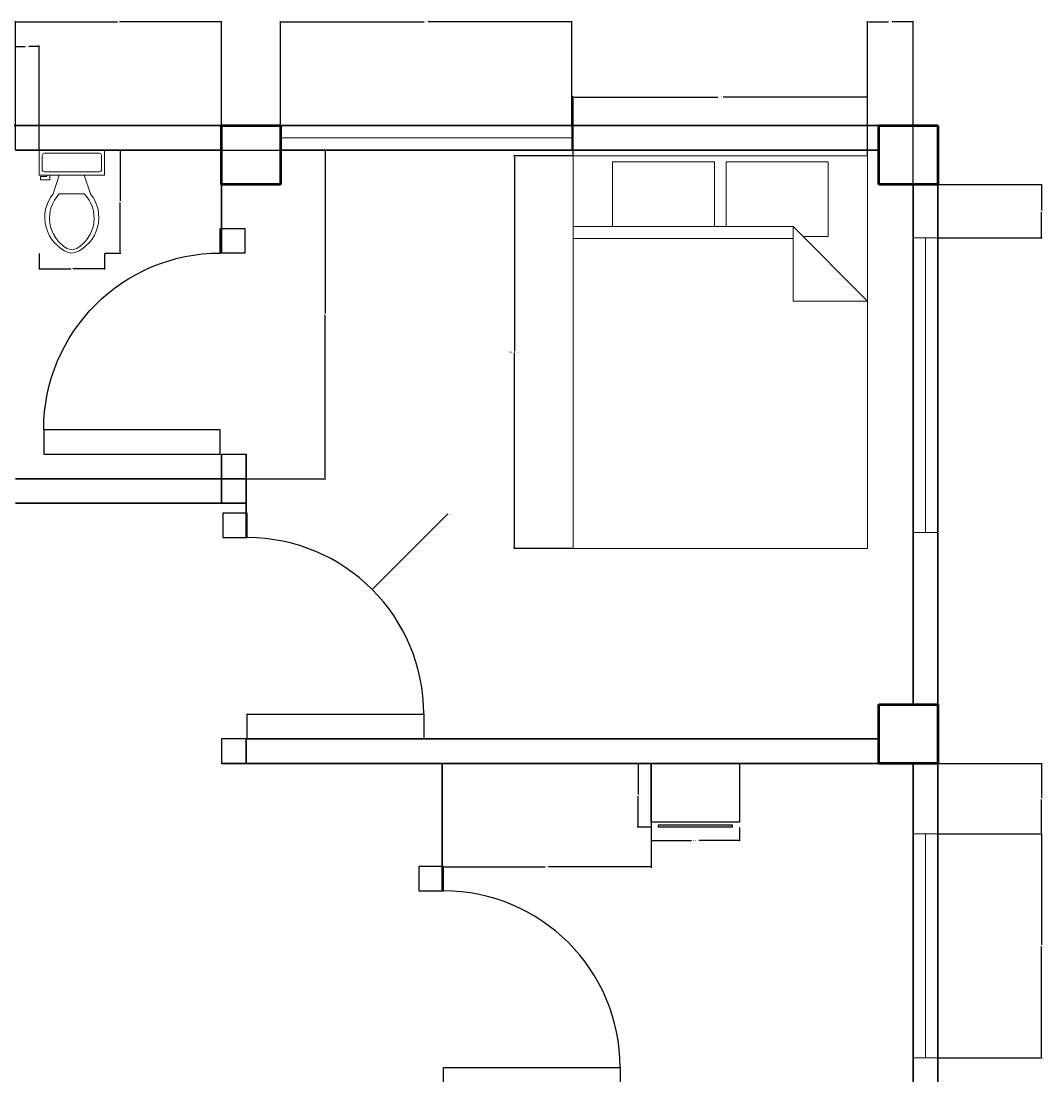
# Model space of a CAD drawing. Units: inches. Extents: x 2082 to 2506, y 790 to 1201.
# Tile 3 of 3: x 2298 to 2506, y 986 to 1201. Entities that reach past the tile are written whole.
import ezdxf

# ---------------------------------------------------------------- set-up
doc = ezdxf.new("R2010")
doc.units = ezdxf.units.IN
for name, color, linetype, lineweight in [('A-ANNO-DIMS', 2, 'Continuous', 18), ('A-COLS', 7, 'Continuous', 50), ('A-DOOR', 3, 'Continuous', 25), ('A-FLOR-CASE', 8, 'Continuous', 25), ('A-FLOR-FIXT', 9, 'Continuous', 18), ('A-FURN', 8, 'Continuous', 18), ('A-GLAZ', 4, 'Continuous', 18), ('A-WALL', 7, 'Continuous', 35)]:
    doc.layers.add(name, color=color, linetype=linetype, lineweight=lineweight)
doc.styles.get("Standard").update_dxf_attribs({"font": 'arial.ttf'})
doc.dimstyles.get("Standard").update_dxf_attribs({"dimtxt": 0.18, "dimasz": 0.18, "dimexe": 0.18, "dimexo": 0.0625, "dimgap": 0.09, "dimtad": 0, "dimtih": 1, "dimtoh": 1, "dimdec": 4, "dimzin": 0, "dimdsep": 46, "dimlunit": 4, "dimtxsty": 'Standard', "dimcen": 0.09, "dimadec": 0, "dimazin": 0, "dimtfac": 1, "dimtdec": 4, "dimtofl": 0, "dimtmove": 0, "dimatfit": 3, "dimfxl": 1, "dimtolj": 1, "dimtzin": 0, "dimarcsym": 0})

# ---------------------------------------------------------------- blocks, each defined once
blk = doc.blocks.new('Wall Cabinet - 18 x 12 in side')
for points in [[(-12, -18), (-12, 0), (0, 0), (0, -18)], [(-13, -16.5), (-13, -1.5), (-12.5, -1.5), (-12.5, -16.5)]]:
    blk.add_lwpolyline(points, close=True)
blk = doc.blocks.new('Toilet - top')
for p, q in [((9.5, -6), (9.5, -2)), ((-10, -8.5), (-8, -8.5)), ((-10, -9.5), (-10, -8.5)), ((-7, -9.5), (-10, -9.5)), ((-8, -8.5), (-8, -8)), ((-7, -8), (-7, -9.5)), ((-4, -8), (-6, -14)), ((4, -8), (6, -14)), ((4, -14), (-4, -14))]:
    blk.add_line(p, q)
blk.add_lwpolyline([(10.5, -8), (10.5, 0), (-10.5, 0), (-10.5, -8)], close=True)
for points in [[(-9.5, -2), (-9.5, -6)], [(8.5, -1), (-8.5, -1)], [(-8.5, -7), (8.5, -7)]]:
    blk.add_lwpolyline(points)
for centre, radius, start, end in [((-8.62, -1.88), 0.884, 81.8699, 188.1301), ((8.62, -1.88), 0.884, 351.8699, 98.1301), ((-8.62, -6.12), 0.884, 171.8699, 278.1301), ((8.62, -6.12), 0.884, 261.8699, 8.1301), ((3.52, -21.58), 12.17, 141.4691, 247.9714), ((4.2, -21.82), 11.33, 136.3677, 238.9468), ((-3.52, -21.58), 12.17, 292.0284, 38.5307), ((-4.2, -21.82), 11.33, 301.053, 43.6321), ((0, -27.88), 4, 245.7318, 294.2682), ((0, -29), 4, 254.8605, 285.1395)]:
    blk.add_arc(centre, radius, start, end)
blk = doc.blocks.new('Bed - Queen')
for p, q in [((0, -80.00003), (0, 0)), ((0, 0), (59.99999, 0)), ((59.99999, 0), (59.99999, -80.00003)), ((7.99999, -1.2), (28.79998, -1.2)), ((7.99999, -14.4), (7.99999, -1.2)), ((28.79998, -1.2), (28.79998, -14.4)), ((31.19999, -1.2), (51.99999, -1.2)), ((31.19999, -14.4), (31.19999, -1.2)), ((51.99999, -1.2), (51.99999, -16.4)), ((0, -14.4), (44.8, -14.4)), ((59.99999, -29.6), (44.8, -14.4)), ((44.8, -14.4), (44.8, -29.6)), ((44.8, -16.8), (0, -16.8)), ((51.99999, -16.4), (46.79936, -16.4)), ((44.8, -29.6), (59.99999, -29.6)), ((59.99999, -80.00003), (0, -80.00003))]:
    blk.add_line(p, q)
blk = doc.blocks.new('DOOR-SWING-36IN')
for p, q in [((0, 0), (0, 5)), ((0, 5), (36, 5)), ((36, 5), (36, 0)), ((36, 0), (0, 0))]:
    blk.add_line(p, q)
blk.add_arc((0, 5), 36, 0, 90)
blk = doc.blocks.new('WIN-60IN')
for p, q in [((0, 5), (12, 5)), ((0, 5), (0, 0)), ((12, 5), (60, 5)), ((60, 5), (60, 0)), ((0, 2.5), (60, 2.5)), ((0, 0), (60, 0))]:
    blk.add_line(p, q)
blk = doc.blocks.new('COL-12X12IN')
for p, q in [((0, 12), (12, 12)), ((0, 0), (0, 12)), ((12, 12), (12, 0)), ((12, 0), (0, 0))]:
    blk.add_line(p, q)
blk = doc.blocks.new('*D10')
at = {"layer": 'A-ANNO-DIMS', "color": 0, "lineweight": -2, "transparency": 16777216}
for p, q in [((2410.56, 1173.3), (2398.44, 1173.3)), ((2398.62, 1173.12), (2398.62, 1133.49)), ((2398.62, 1093.48), (2398.62, 1133.11)), ((2410.56, 1093.3), (2398.44, 1093.3))]:
    blk.add_line(p, q, dxfattribs=at)
at = {"layer": 'A-ANNO-DIMS', "color": 0, "transparency": 16777216}
for points in [[(2398.59, 1173.12), (2398.65, 1173.12), (2398.62, 1173.3)], [(2398.59, 1093.48), (2398.65, 1093.48), (2398.62, 1093.3)]]:
    blk.add_solid(points, dxfattribs=at)
at = {"layer": 'Defpoints', "color": 0, "transparency": 16777216}
for p in [(2398.62, 1173.3), (2410.62, 1173.3), (2410.62, 1093.3)]:
    blk.add_point(p, dxfattribs=at)
at = {"layer": 'A-ANNO-DIMS', "color": 0, "transparency": 16777216, "insert": (2398.62, 1133.3), "char_height": 0.18, "attachment_point": 5}
blk.add_mtext('\\A1;QUEEN BED 80 TYP.', dxfattribs=at)
blk = doc.blocks.new('*D11')
at = {"layer": 'A-ANNO-DIMS', "color": 0, "lineweight": -2, "transparency": 16777216}
for p, q in [((2410.62, 1173.36), (2410.62, 1185.48)), ((2410.8, 1185.3), (2440.09, 1185.3)), ((2470.44, 1185.3), (2441.15, 1185.3)), ((2470.62, 1173.36), (2470.62, 1185.48))]:
    blk.add_line(p, q, dxfattribs=at)
at = {"layer": 'A-ANNO-DIMS', "color": 0, "transparency": 16777216}
for points in [[(2410.8, 1185.33), (2410.8, 1185.27), (2410.62, 1185.3)], [(2470.44, 1185.33), (2470.44, 1185.27), (2470.62, 1185.3)]]:
    blk.add_solid(points, dxfattribs=at)
at = {"layer": 'Defpoints', "color": 0, "transparency": 16777216}
for p in [(2470.62, 1185.3), (2410.62, 1173.3), (2470.62, 1173.3)]:
    blk.add_point(p, dxfattribs=at)
at = {"layer": 'A-ANNO-DIMS', "color": 0, "transparency": 16777216, "insert": (2440.62, 1185.3), "char_height": 0.18, "attachment_point": 5}
blk.add_mtext('\\A1;60 TYP.', dxfattribs=at)
blk = doc.blocks.new('*D18')
at = {"layer": 'A-ANNO-DIMS', "color": 0, "lineweight": -2, "transparency": 16777216}
for p, q in [((2315.16, 1174.5), (2318.43, 1174.5)), ((2318.25, 1174.32), (2318.25, 1164.17)), ((2318.25, 1153.65), (2318.25, 1163.8)), ((2315.16, 1153.47), (2318.43, 1153.47))]:
    blk.add_line(p, q, dxfattribs=at)
at = {"layer": 'A-ANNO-DIMS', "color": 0, "transparency": 16777216}
for points in [[(2318.22, 1174.32), (2318.28, 1174.32), (2318.25, 1174.5)], [(2318.22, 1153.65), (2318.28, 1153.65), (2318.25, 1153.47)]]:
    blk.add_solid(points, dxfattribs=at)
at = {"layer": 'Defpoints', "color": 0, "transparency": 16777216}
for p in [(2315.09, 1174.5), (2318.25, 1174.5), (2315.09, 1153.47)]:
    blk.add_point(p, dxfattribs=at)
at = {"layer": 'A-ANNO-DIMS', "color": 0, "transparency": 16777216, "insert": (2318.25, 1163.98), "char_height": 0.18, "attachment_point": 5}
blk.add_mtext('\\A1;WC 21', dxfattribs=at)
blk = doc.blocks.new('*D19')
at = {"layer": 'A-ANNO-DIMS', "color": 0, "lineweight": -2, "transparency": 16777216}
for p, q in [((2301.73, 1153.4), (2301.73, 1150.13)), ((2315.09, 1153.4), (2315.09, 1150.13)), ((2301.91, 1150.31), (2308.2, 1150.31)), ((2314.91, 1150.31), (2308.62, 1150.31))]:
    blk.add_line(p, q, dxfattribs=at)
at = {"layer": 'A-ANNO-DIMS', "color": 0, "transparency": 16777216}
for points in [[(2301.91, 1150.34), (2301.91, 1150.28), (2301.73, 1150.31)], [(2314.91, 1150.34), (2314.91, 1150.28), (2315.09, 1150.31)]]:
    blk.add_solid(points, dxfattribs=at)
at = {"layer": 'Defpoints', "color": 0, "transparency": 16777216}
for p in [(2301.73, 1153.47), (2315.09, 1153.47), (2315.09, 1150.31)]:
    blk.add_point(p, dxfattribs=at)
at = {"layer": 'A-ANNO-DIMS', "color": 0, "transparency": 16777216, "insert": (2308.41, 1150.31), "char_height": 0.18, "attachment_point": 5}
blk.add_mtext('\\A1;13', dxfattribs=at)
blk = doc.blocks.new('*D20')
at = {"layer": 'A-ANNO-DIMS', "color": 0, "lineweight": -2, "transparency": 16777216}
for p, q in [((2426.53, 1036.44), (2426.53, 1033.62)), ((2444.53, 1036.44), (2444.53, 1033.62)), ((2426.71, 1033.8), (2434.73, 1033.8)), ((2444.35, 1033.8), (2436.32, 1033.8))]:
    blk.add_line(p, q, dxfattribs=at)
at = {"layer": 'A-ANNO-DIMS', "color": 0, "transparency": 16777216}
for points in [[(2426.71, 1033.83), (2426.71, 1033.77), (2426.53, 1033.8)], [(2444.35, 1033.83), (2444.35, 1033.77), (2444.53, 1033.8)]]:
    blk.add_solid(points, dxfattribs=at)
at = {"layer": 'Defpoints', "color": 0, "transparency": 16777216}
for p in [(2426.53, 1036.5), (2444.53, 1036.5), (2426.53, 1033.8)]:
    blk.add_point(p, dxfattribs=at)
at = {"layer": 'A-ANNO-DIMS', "color": 0, "transparency": 16777216, "insert": (2435.53, 1033.8), "char_height": 0.18, "attachment_point": 5}
blk.add_mtext('\\A1;CABINET 18', dxfattribs=at)
blk = doc.blocks.new('*D21')
at = {"layer": 'A-ANNO-DIMS', "color": 0, "lineweight": -2, "transparency": 16777216}
for p, q in [((2426.46, 1049.5), (2423.65, 1049.5)), ((2423.83, 1049.32), (2423.83, 1043.18)), ((2423.83, 1036.68), (2423.83, 1042.82)), ((2426.46, 1036.5), (2423.65, 1036.5))]:
    blk.add_line(p, q, dxfattribs=at)
at = {"layer": 'A-ANNO-DIMS', "color": 0, "transparency": 16777216}
for points in [[(2423.8, 1049.32), (2423.86, 1049.32), (2423.83, 1049.5)], [(2423.8, 1036.68), (2423.86, 1036.68), (2423.83, 1036.5)]]:
    blk.add_solid(points, dxfattribs=at)
at = {"layer": 'Defpoints', "color": 0, "transparency": 16777216}
for p in [(2423.83, 1049.5), (2426.53, 1049.5), (2426.53, 1036.5)]:
    blk.add_point(p, dxfattribs=at)
at = {"layer": 'A-ANNO-DIMS', "color": 0, "transparency": 16777216, "insert": (2423.83, 1043), "char_height": 0.18, "attachment_point": 5}
blk.add_mtext('\\A1;13', dxfattribs=at)
blk = doc.blocks.new('*D33')
at = {"layer": 'A-ANNO-DIMS', "color": 0, "lineweight": -2, "transparency": 16777216}
for p, q in [((2296.92, 1174.56), (2296.92, 1200.78)), ((2338.92, 1174.56), (2338.92, 1200.78)), ((2297.1, 1200.6), (2317.7, 1200.6)), ((2338.74, 1200.6), (2318.15, 1200.6))]:
    blk.add_line(p, q, dxfattribs=at)
at = {"layer": 'A-ANNO-DIMS', "color": 0, "transparency": 16777216}
for points in [[(2297.1, 1200.63), (2297.1, 1200.57), (2296.92, 1200.6)], [(2338.74, 1200.63), (2338.74, 1200.57), (2338.92, 1200.6)]]:
    blk.add_solid(points, dxfattribs=at)
at = {"layer": 'Defpoints', "color": 0, "transparency": 16777216}
for p in [(2338.92, 1200.6), (2296.92, 1174.5), (2338.92, 1174.5)]:
    blk.add_point(p, dxfattribs=at)
at = {"layer": 'A-ANNO-DIMS', "color": 0, "transparency": 16777216, "insert": (2317.92, 1200.6), "char_height": 0.18, "attachment_point": 5}
blk.add_mtext('\\A1;42', dxfattribs=at)
blk = doc.blocks.new('*D34')
at = {"layer": 'A-ANNO-DIMS', "color": 0, "lineweight": -2, "transparency": 16777216}
for p, q in [((2350.92, 1179.56), (2350.92, 1200.78)), ((2410.34, 1179.56), (2410.34, 1200.78)), ((2351.1, 1200.6), (2380.24, 1200.6)), ((2410.16, 1200.6), (2381.02, 1200.6))]:
    blk.add_line(p, q, dxfattribs=at)
at = {"layer": 'A-ANNO-DIMS', "color": 0, "transparency": 16777216}
for points in [[(2351.1, 1200.63), (2351.1, 1200.57), (2350.92, 1200.6)], [(2410.16, 1200.63), (2410.16, 1200.57), (2410.34, 1200.6)]]:
    blk.add_solid(points, dxfattribs=at)
at = {"layer": 'Defpoints', "color": 0, "transparency": 16777216}
for p in [(2410.34, 1200.6), (2350.92, 1179.5), (2410.34, 1179.5)]:
    blk.add_point(p, dxfattribs=at)
at = {"layer": 'A-ANNO-DIMS', "color": 0, "transparency": 16777216, "insert": (2380.63, 1200.6), "char_height": 0.18, "attachment_point": 5}
blk.add_mtext('\\A1;59.42', dxfattribs=at)
blk = doc.blocks.new('*D35')
at = {"layer": 'A-ANNO-DIMS', "color": 0, "lineweight": -2, "transparency": 16777216}
for p, q in [((2338.99, 1174.5), (2360.2, 1174.5)), ((2360.02, 1174.32), (2360.02, 1141.18)), ((2360.02, 1107.68), (2360.02, 1140.82)), ((2338.99, 1107.5), (2360.2, 1107.5))]:
    blk.add_line(p, q, dxfattribs=at)
at = {"layer": 'A-ANNO-DIMS', "color": 0, "transparency": 16777216}
for points in [[(2359.99, 1174.32), (2360.05, 1174.32), (2360.02, 1174.5)], [(2359.99, 1107.68), (2360.05, 1107.68), (2360.02, 1107.5)]]:
    blk.add_solid(points, dxfattribs=at)
at = {"layer": 'Defpoints', "color": 0, "transparency": 16777216}
for p in [(2338.92, 1174.5), (2338.92, 1107.5), (2360.02, 1107.5)]:
    blk.add_point(p, dxfattribs=at)
at = {"layer": 'A-ANNO-DIMS', "color": 0, "transparency": 16777216, "insert": (2360.02, 1141), "char_height": 0.18, "attachment_point": 5}
blk.add_mtext('\\A1;67', dxfattribs=at)
blk = doc.blocks.new('*D44')
at = {"layer": 'A-ANNO-DIMS', "color": 0, "lineweight": -2, "transparency": 16777216}
for p, q in [((2484.99, 1167.5), (2506.23, 1167.5)), ((2506.05, 1167.32), (2506.05, 1162.22)), ((2506.05, 1156.75), (2506.05, 1161.85)), ((2484.99, 1156.57), (2506.23, 1156.57))]:
    blk.add_line(p, q, dxfattribs=at)
at = {"layer": 'A-ANNO-DIMS', "color": 0, "transparency": 16777216}
for points in [[(2506.02, 1167.32), (2506.08, 1167.32), (2506.05, 1167.5)], [(2506.02, 1156.75), (2506.08, 1156.75), (2506.05, 1156.57)]]:
    blk.add_solid(points, dxfattribs=at)
at = {"layer": 'Defpoints', "color": 0, "transparency": 16777216}
for p in [(2484.92, 1167.5), (2506.05, 1167.5), (2484.92, 1156.57)]:
    blk.add_point(p, dxfattribs=at)
at = {"layer": 'A-ANNO-DIMS', "color": 0, "transparency": 16777216, "insert": (2506.05, 1162.03), "char_height": 0.18, "attachment_point": 5}
blk.add_mtext('\\A1;10.93', dxfattribs=at)
blk = doc.blocks.new('*D45')
at = {"layer": 'A-ANNO-DIMS', "color": 0, "lineweight": -2, "transparency": 16777216}
for p, q in [((2484.99, 1035.14), (2506.23, 1035.14)), ((2506.05, 1034.96), (2506.05, 1012.5)), ((2506.05, 989.68), (2506.05, 1012.14)), ((2484.99, 989.5), (2506.23, 989.5))]:
    blk.add_line(p, q, dxfattribs=at)
at = {"layer": 'A-ANNO-DIMS', "color": 0, "transparency": 16777216}
for points in [[(2506.02, 1034.96), (2506.08, 1034.96), (2506.05, 1035.14)], [(2506.02, 989.68), (2506.08, 989.68), (2506.05, 989.5)]]:
    blk.add_solid(points, dxfattribs=at)
at = {"layer": 'Defpoints', "color": 0, "transparency": 16777216}
for p in [(2484.92, 1035.14), (2506.05, 1035.14), (2484.92, 989.5)]:
    blk.add_point(p, dxfattribs=at)
at = {"layer": 'A-ANNO-DIMS', "color": 0, "transparency": 16777216, "insert": (2506.05, 1012.32), "char_height": 0.18, "attachment_point": 5}
blk.add_mtext('\\A1;45.64', dxfattribs=at)
blk = doc.blocks.new('*D46')
at = {"layer": 'A-ANNO-DIMS', "color": 0, "lineweight": -2, "transparency": 16777216}
for p, q in [((2484.99, 1049.48), (2506.23, 1049.48)), ((2506.05, 1049.3), (2506.05, 1042.49)), ((2506.05, 1035.32), (2506.05, 1042.12)), ((2484.99, 1035.14), (2506.23, 1035.14))]:
    blk.add_line(p, q, dxfattribs=at)
at = {"layer": 'A-ANNO-DIMS', "color": 0, "transparency": 16777216}
for points in [[(2506.02, 1049.3), (2506.08, 1049.3), (2506.05, 1049.48)], [(2506.02, 1035.32), (2506.08, 1035.32), (2506.05, 1035.14)]]:
    blk.add_solid(points, dxfattribs=at)
at = {"layer": 'Defpoints', "color": 0, "transparency": 16777216}
for p in [(2484.92, 1049.48), (2506.05, 1049.48), (2484.92, 1035.14)]:
    blk.add_point(p, dxfattribs=at)
at = {"layer": 'A-ANNO-DIMS', "color": 0, "transparency": 16777216, "insert": (2506.05, 1042.31), "char_height": 0.18, "attachment_point": 5}
blk.add_mtext('\\A1;14.34', dxfattribs=at)
blk = doc.blocks.new('*D48')
at = {"layer": 'A-ANNO-DIMS', "color": 0, "lineweight": -2, "transparency": 16777216}
for p, q in [((2383.92, 1049.44), (2383.92, 1028.22)), ((2426.53, 1049.44), (2426.53, 1028.22)), ((2384.1, 1028.4), (2404.9, 1028.4)), ((2426.35, 1028.4), (2405.55, 1028.4))]:
    blk.add_line(p, q, dxfattribs=at)
at = {"layer": 'A-ANNO-DIMS', "color": 0, "transparency": 16777216}
for points in [[(2384.1, 1028.43), (2384.1, 1028.37), (2383.92, 1028.4)], [(2426.35, 1028.43), (2426.35, 1028.37), (2426.53, 1028.4)]]:
    blk.add_solid(points, dxfattribs=at)
at = {"layer": 'Defpoints', "color": 0, "transparency": 16777216}
for p in [(2383.92, 1049.5), (2426.53, 1049.5), (2383.92, 1028.4)]:
    blk.add_point(p, dxfattribs=at)
at = {"layer": 'A-ANNO-DIMS', "color": 0, "transparency": 16777216, "insert": (2405.22, 1028.4), "char_height": 0.18, "attachment_point": 5}
blk.add_mtext('\\A1;42.6', dxfattribs=at)
blk = doc.blocks.new('*D50')
at = {"layer": 'A-ANNO-DIMS', "color": 0, "lineweight": -2, "transparency": 16777216}
for p, q in [((2470.62, 1173.36), (2470.62, 1200.78)), ((2479.92, 1167.56), (2479.92, 1200.78)), ((2470.8, 1200.6), (2474.88, 1200.6)), ((2479.74, 1200.6), (2475.66, 1200.6))]:
    blk.add_line(p, q, dxfattribs=at)
at = {"layer": 'A-ANNO-DIMS', "color": 0, "transparency": 16777216}
for points in [[(2470.8, 1200.63), (2470.8, 1200.57), (2470.62, 1200.6)], [(2479.74, 1200.63), (2479.74, 1200.57), (2479.92, 1200.6)]]:
    blk.add_solid(points, dxfattribs=at)
at = {"layer": 'Defpoints', "color": 0, "transparency": 16777216}
for p in [(2479.92, 1200.6), (2470.62, 1173.3), (2479.92, 1167.5)]:
    blk.add_point(p, dxfattribs=at)
at = {"layer": 'A-ANNO-DIMS', "color": 0, "transparency": 16777216, "insert": (2475.27, 1200.6), "char_height": 0.18, "attachment_point": 5}
blk.add_mtext('\\A1;9.306', dxfattribs=at)
blk = doc.blocks.new('*D53')
at = {"layer": 'A-ANNO-DIMS', "color": 0, "lineweight": -2, "transparency": 16777216}
for p, q in [((2296.92, 1174.56), (2296.92, 1195.78)), ((2297.1, 1195.6), (2298.93, 1195.6)), ((2301.55, 1195.6), (2299.72, 1195.6)), ((2301.73, 1174.56), (2301.73, 1195.78))]:
    blk.add_line(p, q, dxfattribs=at)
at = {"layer": 'A-ANNO-DIMS', "color": 0, "transparency": 16777216}
for points in [[(2297.1, 1195.63), (2297.1, 1195.57), (2296.92, 1195.6)], [(2301.55, 1195.63), (2301.55, 1195.57), (2301.73, 1195.6)]]:
    blk.add_solid(points, dxfattribs=at)
at = {"layer": 'Defpoints', "color": 0, "transparency": 16777216}
for p in [(2301.73, 1195.6), (2296.92, 1174.5), (2301.73, 1174.5)]:
    blk.add_point(p, dxfattribs=at)
at = {"layer": 'A-ANNO-DIMS', "color": 0, "transparency": 16777216, "insert": (2299.33, 1195.6), "char_height": 0.18, "attachment_point": 5}
blk.add_mtext('\\A1;4.805', dxfattribs=at)
blk = doc.blocks.new('*D57')
at = {"layer": 'A-ANNO-DIMS', "color": 0, "lineweight": -2, "transparency": 16777216}
for p, q in [((2384.9, 1100.23), (2369.75, 1085.08)), ((2385.08, 1100.23), (2384.9, 1100.23)), ((2344.08, 1059.5), (2344.26, 1059.5)), ((2344.17, 1059.41), (2344.17, 1059.59))]:
    blk.add_line(p, q, dxfattribs=at)
at = {"layer": 'A-ANNO-DIMS', "color": 0, "transparency": 16777216}
blk.add_solid([(2369.73, 1085.1), (2369.77, 1085.06), (2369.63, 1084.96)], dxfattribs=at)
at = {"layer": 'Defpoints', "color": 0, "transparency": 16777216}
for p in [(2369.63, 1084.96), (2344.17, 1059.5)]:
    blk.add_point(p, dxfattribs=at)
at = {"layer": 'A-ANNO-DIMS', "color": 0, "transparency": 16777216, "insert": (2385.58, 1100.23), "char_height": 0.18, "attachment_point": 5}
blk.add_mtext('\\A1;6X R36', dxfattribs=at)

msp = doc.modelspace()

# ---------------------------------------------------------------- linework, layer by layer
at = {"layer": 'A-DOOR'}
for p, q in [((2338.6767, 1153.4988), (2338.6767, 1158.4988)), ((2338.6767, 1158.4988), (2343.6767, 1158.4988)), ((2343.6767, 1158.4988), (2343.6767, 1153.4988)), ((2343.6767, 1153.4988), (2338.6767, 1153.4988)), ((2338.9236, 1107.4988), (2338.9236, 1112.4988)), ((2338.9236, 1112.4988), (2343.9236, 1112.4988)), ((2343.8994, 1112.4988), (2343.9236, 1107.4988)), ((2343.9236, 1107.4988), (2338.9236, 1107.4988)), ((2339.1705, 1100.4988), (2339.1705, 1095.4988)), ((2344.1705, 1100.4988), (2339.1705, 1100.4988)), ((2344.1705, 1095.4988), (2344.1705, 1100.4988)), ((2339.1705, 1095.4988), (2344.1705, 1095.4988)), ((2338.9236, 1054.4988), (2338.9236, 1049.4988)), ((2343.9236, 1054.4988), (2338.9236, 1054.4988)), ((2338.9236, 1054.4988), (2338.9236, 1049.4988)), ((2343.9236, 1049.4988), (2343.9236, 1054.4988)), ((2343.9236, 1054.4988), (2343.9236, 1049.4988)), ((2338.9236, 1049.4988), (2343.9236, 1049.4988)), ((2379.1705, 1028.4988), (2379.1705, 1023.4988)), ((2384.1705, 1028.4988), (2379.1705, 1028.4988)), ((2384.1705, 1023.4988), (2384.1705, 1028.4988)), ((2379.1705, 1023.4988), (2384.1705, 1023.4988))]:
    msp.add_line(p, q, dxfattribs=at)
at = {"layer": 'A-GLAZ'}
for p, q in [((2350.34, 1179.4988), (2362.34, 1179.4988)), ((2362.34, 1179.4988), (2410.34, 1179.4988)), ((2410.34, 1179.4988), (2410.34, 1174.4988)), ((2350.9161, 1176.9988), (2410.34, 1176.9988)), ((2350.9161, 1174.4988), (2410.34, 1174.4988)), ((2479.9236, 1049.4988), (2479.9236, 989.4988)), ((2484.9236, 1049.4988), (2484.9236, 1037.4988)), ((2484.9236, 1037.4988), (2484.9236, 989.4988)), ((2479.9236, 1035.1356), (2484.9236, 1035.1356)), ((2482.4236, 1035.1356), (2482.4236, 989.4988)), ((2484.9236, 989.4988), (2479.9236, 989.4988))]:
    msp.add_line(p, q, dxfattribs=at)
at = {"layer": 'A-WALL'}
for p, q in [((2107.9236, 1179.4988), (2479.9236, 1179.4988)), ((2479.9236, 1179.4988), (2484.9236, 1179.4988)), ((2484.9236, 1179.4988), (2484.9236, 850.4988)), ((2338.9236, 1174.4988), (2296.9236, 1174.4988)), ((2338.9236, 1153.4988), (2338.9236, 1174.4988)), ((2472.9246, 1174.4988), (2350.9161, 1174.4988)), ((2350.9161, 1174.4988), (2472.9246, 1174.4988)), ((2479.9236, 1061.4755), (2479.9236, 1167.4988)), ((2479.9236, 1167.4988), (2479.9236, 1061.4755)), ((2338.9236, 1107.4988), (2338.9236, 1112.4988)), ((2343.9236, 1107.4988), (2343.9236, 1112.4988)), ((2296.9236, 1107.4988), (2343.9236, 1107.4988)), ((2338.9236, 1107.4988), (2338.9236, 1102.4988)), ((2343.9236, 1107.4988), (2343.9236, 1095.4988)), ((2296.9236, 1102.4988), (2343.9236, 1102.4988)), ((2364.9236, 1054.4988), (2343.9236, 1054.4988)), ((2472.9226, 1054.4988), (2364.9236, 1054.4988)), ((2338.9236, 1049.4988), (2343.9236, 1049.4988)), ((2364.9236, 1049.4988), (2343.9236, 1049.4988)), ((2479.9236, 1049.4988), (2364.9236, 1049.4988)), ((2479.9236, 1049.4988), (2383.9236, 1049.4988)), ((2383.9236, 1049.4988), (2383.9236, 1023.4988)), ((2479.9236, 977.4988), (2479.9236, 1049.4988))]:
    msp.add_line(p, q, dxfattribs=at)

# ---------------------------------------------------------------- block references
at = {"layer": 'A-COLS'}
for p, rotation in [((2350.9161, 1167.4988), 90.00000000000216), ((2484.9246, 1167.4988), 90.00000000000216), ((2484.9226, 1049.4755), 90.00000000000325)]:
    msp.add_blockref('COL-12X12IN', p, dxfattribs=dict(at, rotation=rotation))
at = {"layer": 'A-DOOR', "extrusion": (0, 0, -1), "zscale": -1}
msp.add_blockref('DOOR-SWING-36IN', (-2338.6767, 1112.4988), dxfattribs=at)
at = {"layer": 'A-DOOR'}
for p in [(2344.1705, 1054.4988), (2384.1705, 982.4988)]:
    msp.add_blockref('DOOR-SWING-36IN', p, dxfattribs=at)
at = {"layer": 'A-FLOR-CASE', "rotation": 90}
msp.add_blockref('Wall Cabinet - 18 x 12 in side', (2426.5256, 1049.4988), dxfattribs=at)
at = {"layer": 'A-FLOR-FIXT', "xscale": 0.6364643195788697, "yscale": 0.6364643195788697, "zscale": 0.6364643195788697}
msp.add_blockref('Toilet - top', (2308.4112, 1174.4988), dxfattribs=at)
at = {"layer": 'A-FURN'}
msp.add_blockref('Bed - Queen', (2410.6176, 1173.2988), dxfattribs=at)
at = {"layer": 'A-GLAZ', "rotation": 269.9999999999998}
msp.add_blockref('WIN-60IN', (2479.9236, 1156.569), dxfattribs=at)

# ---------------------------------------------------------------- dimensions: what is measured, and where the dimension line sits
at = {"layer": 'A-ANNO-DIMS'}
for base, p1, p2, override, picture, middle in [((2338.9236, 1200.5988), (2296.9236, 1174.4988), (2338.9236, 1174.4988), {"dimdec": 0, "dimlfac": 1, "dimrnd": 0, "dimzin": 0, "dimdsep": 46, "dimlunit": 2}, '*D33', (2317.9236, 1200.5988)), ((2410.34, 1200.5988), (2350.9161, 1179.4988), (2410.34, 1179.4988), {"dimdec": 2, "dimlfac": 1, "dimrnd": 0, "dimzin": 0, "dimdsep": 46, "dimlunit": 2}, '*D34', (2380.628, 1200.5988)), ((2479.9236, 1200.5988), (2470.6175, 1173.2988), (2479.9236, 1167.4988), {"dimdec": 3, "dimlfac": 1, "dimrnd": 0, "dimzin": 0, "dimdsep": 46, "dimlunit": 2}, '*D50', (2475.2706, 1200.5988)), ((2301.7283, 1195.5988), (2296.9236, 1174.4988), (2301.7283, 1174.4988), {"dimdec": 3, "dimlfac": 1, "dimrnd": 0, "dimzin": 0, "dimdsep": 46, "dimlunit": 2}, '*D53', (2299.326, 1195.5988)), ((2315.094, 1150.3112), (2301.7283, 1153.4661), (2315.094, 1153.4661), {"dimdec": 0, "dimlfac": 1, "dimrnd": 0, "dimzin": 0, "dimdsep": 46, "dimlunit": 2}, '*D19', (2308.4112, 1150.3112))]:
    dim = msp.add_linear_dim(base=base, p1=p1, p2=p2, dimstyle='Standard', override=override, dxfattribs=at)
    dim.commit()
    dim.dimension.update_dxf_attribs({"geometry": picture, "text_midpoint": middle})
dim = msp.add_linear_dim(base=(2470.6175, 1185.2988), p1=(2410.6176, 1173.2988), p2=(2470.6175, 1173.2988), text='<> TYP.', dimstyle='Standard', override={"dimdec": 0, "dimlfac": 1, "dimrnd": 0, "dimzin": 0, "dimdsep": 46, "dimlunit": 2}, dxfattribs=at)
dim.commit()
dim.dimension.update_dxf_attribs({"geometry": '*D11', "text_midpoint": (2440.6175, 1185.2988)})
for base, p1, p2, angle, text, picture, middle in [((2318.2489, 1174.4988), (2315.094, 1153.4661), (2315.094, 1174.4988), 90, 'WC <>', '*D18', (2318.2489, 1163.9825)), ((2398.6175, 1173.2988), (2410.6176, 1093.2988), (2410.6176, 1173.2988), 90, 'QUEEN BED <> TYP.', '*D10', (2398.6175, 1133.2988)), ((2426.5256, 1033.7988), (2444.5256, 1036.4988), (2426.5256, 1036.4988), 180, 'CABINET <>', '*D20', (2435.5256, 1033.7988))]:
    dim = msp.add_linear_dim(base=base, p1=p1, p2=p2, angle=angle, text=text, dimstyle='Standard', override={"dimdec": 0, "dimlfac": 1, "dimrnd": 0, "dimzin": 0, "dimdsep": 46, "dimlunit": 2}, dxfattribs=at)
    dim.commit()
    dim.dimension.update_dxf_attribs({"geometry": picture, "text_midpoint": middle})
for base, p1, p2, angle, override, picture, middle in [((2360.0236, 1107.4988), (2338.9236, 1174.4988), (2338.9236, 1107.4988), 270, {"dimdec": 0, "dimlfac": 1, "dimrnd": 0, "dimzin": 0, "dimdsep": 46, "dimlunit": 2}, '*D35', (2360.0236, 1140.9988)), ((2506.0535, 1167.4988), (2484.9236, 1156.569), (2484.9246, 1167.4988), 90, {"dimdec": 2, "dimlfac": 1, "dimrnd": 0, "dimzin": 0, "dimdsep": 46, "dimlunit": 2}, '*D44', (2506.0535, 1162.0339)), ((2383.9236, 1028.3988), (2426.5256, 1049.4988), (2383.9236, 1049.4988), 180, {"dimdec": 1, "dimlfac": 1, "dimrnd": 0, "dimzin": 0, "dimdsep": 46, "dimlunit": 2}, '*D48', (2405.2246, 1028.3988)), ((2423.8256, 1049.4988), (2426.5256, 1036.4988), (2426.5256, 1049.4988), 90, {"dimdec": 0, "dimlfac": 1, "dimrnd": 0, "dimzin": 0, "dimdsep": 46, "dimlunit": 2}, '*D21', (2423.8256, 1042.9988)), ((2506.0535, 1049.4755), (2484.9236, 1035.1356), (2484.9226, 1049.4755), 90, {"dimdec": 2, "dimlfac": 1, "dimrnd": 0, "dimzin": 0, "dimdsep": 46, "dimlunit": 2}, '*D46', (2506.0535, 1042.3055)), ((2506.0535, 1035.1356), (2484.9236, 989.4988), (2484.9236, 1035.1356), 90, {"dimdec": 2, "dimlfac": 1, "dimrnd": 0, "dimzin": 0, "dimdsep": 46, "dimlunit": 2}, '*D45', (2506.0535, 1012.3172))]:
    dim = msp.add_linear_dim(base=base, p1=p1, p2=p2, angle=angle, dimstyle='Standard', override=override, dxfattribs=at)
    dim.commit()
    dim.dimension.update_dxf_attribs({"geometry": picture, "text_midpoint": middle})
dim = msp.add_radius_dim(center=(2344.1705, 1059.4988), mpoint=(2369.626, 1084.955), text='6X <>', dimstyle='Standard', override={"dimdec": 0, "dimlfac": 1, "dimrnd": 0, "dimzin": 0, "dimdsep": 46, "dimlunit": 2}, dxfattribs=at)
dim.commit()
dim.dimension.update_dxf_attribs({"geometry": '*D57', "text_midpoint": (2385.5782, 1100.2287), "dimtype": 164})

doc.saveas('drawing.dxf')
